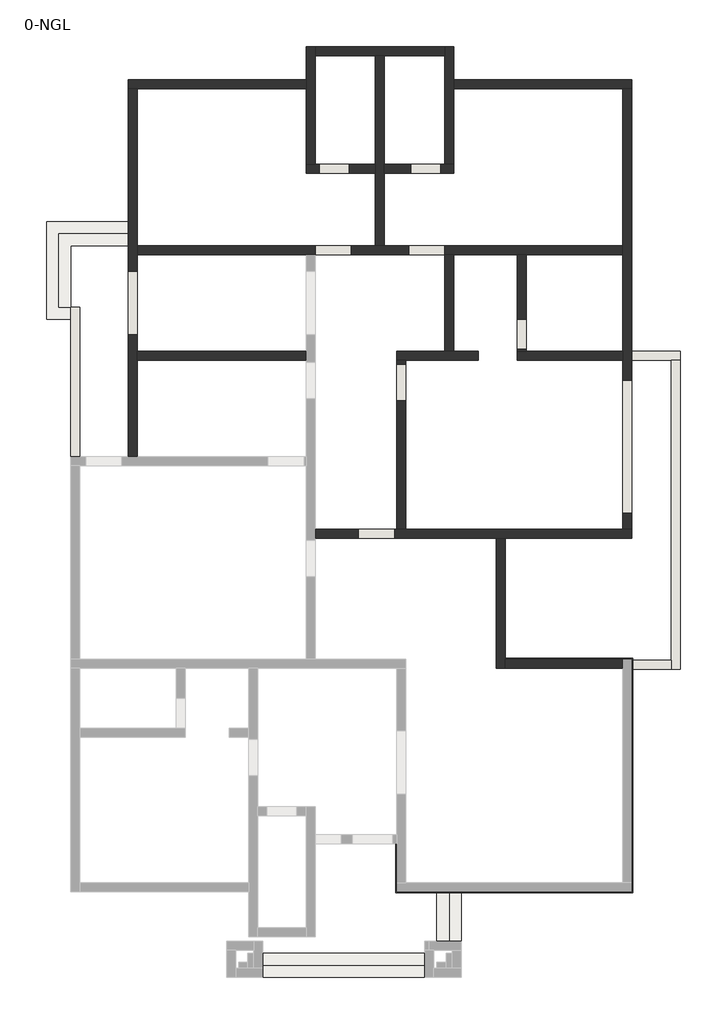
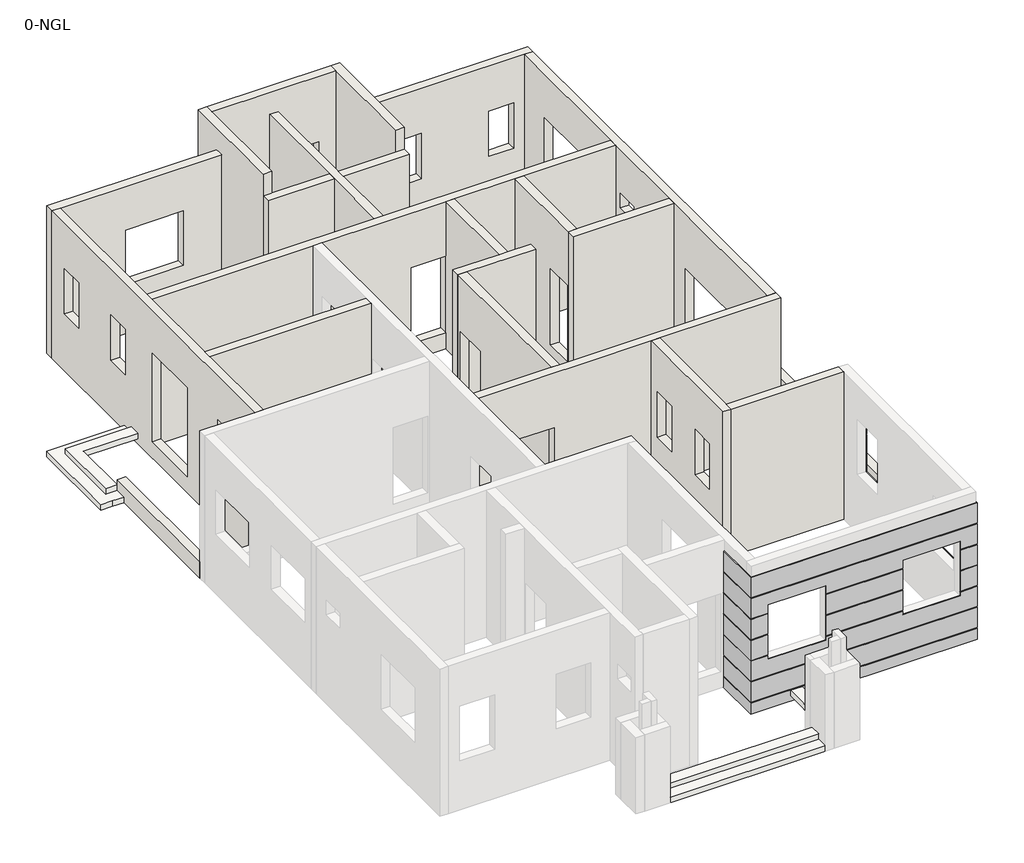
# One storey, part 2 of 2: 23 walls, 4 slabs, 1 furniture element.
"""IFC4 building model written with IfcOpenShell, lengths in millimetres."""

from ifc_helpers import new_model, si_unit, frame, origin, origin_with_axes, place, context, project, spatial, polyline, outline, extrude, faceted_brep, transform, mapped, element, save
from components import casework_8_casework_8_de918fe4

model = new_model("IFC4")

# Units and contexts
model_context = context("Model", 3, world=origin())
ifc_project = project(units=[si_unit("LENGTHUNIT", "METRE", prefix="MILLI")], contexts=[model_context])

# Site, building, storey
site = spatial("IfcSite", under=ifc_project)
building = spatial("IfcBuilding", under=site)
storey = spatial("IfcBuildingStorey", under=building, Name="0-NGL", Elevation=0.0)

# Furniture
placement = place(None, origin())
casework_8_casework_8_shape = casework_8_casework_8_de918fe4(model_context)
element("IfcFurniture", 1, ObjectType="Casework 8 : Casework 8", at=placement, inside=storey, context=model_context, shape_type="MappedRepresentation", body=[
    mapped(casework_8_casework_8_shape, transform((0.0, 0.0, 0.0), x_axis=(1.0, 0.0, 0.0), y_axis=(0.0, 1.0, 0.0), z_axis=(0.0, 0.0, 1.0))),
])

# Slabs
element("IfcSlab", 2, ObjectType="6\" floor", at=placement, inside=storey, context=model_context, shape_type="SweptSolid", body=[
    extrude(outline(polyline([(-6111.7953966, 4965.8070837), (-6111.7953966, 3440.8070837), (-6411.7953966, 3440.8070837), (-6411.7953966, 5265.8070837), (-4686.7953966, 5265.8070837), (-4686.7953966, 4965.8070837), (-6111.7953966, 4965.8070837)])), frame((0.0, 0.0, 150.0), z_axis=(0.0, 0.0, 1.0), x_axis=(1.0, 0.0, 0.0)), (0.0, 0.0, 1.0), 150.0),
])
element("IfcSlab", 3, ObjectType="6\" floor", at=placement, inside=storey, context=model_context, shape_type="SweptSolid", body=[
    extrude(outline(polyline([(-6411.7953966, 5265.8070837), (-6411.7953966, 3440.8070837), (-6111.7953966, 3440.8070837), (-6111.7953966, 3140.8070837), (-6411.7953966, 3140.8070837), (-6711.7953966, 3140.8070837), (-6711.7953966, 5565.8070837), (-4686.7953966, 5565.8070837), (-4686.7953966, 5265.8070837), (-6411.7953966, 5265.8070837)])), origin_with_axes(), (0.0, 0.0, 1.0), 150.0),
])
element("IfcSlab", 4, ObjectType="6\" floor", at=placement, inside=storey, context=model_context, shape_type="SweptSolid", body=[
    extrude(outline(polyline([(2993.2046034, -11134.1929163), (3293.2046034, -11134.1929163), (3293.2046034, -12324.1929163), (2993.2046034, -12324.1929163), (2993.2046034, -11134.1929163)])), frame((0.0, 0.0, 150.0), z_axis=(0.0, 0.0, 1.0), x_axis=(1.0, 0.0, 0.0)), (0.0, 0.0, 1.0), 150.0),
    extrude(outline(polyline([(2693.2046034, -12624.1929163), (2693.2046034, -12924.1929163), (-1336.7953966, -12924.1929163), (-1336.7953966, -12624.1929163), (2693.2046034, -12624.1929163)])), frame((0.0, 0.0, 150.0), z_axis=(0.0, 0.0, 1.0), x_axis=(1.0, 0.0, 0.0)), (0.0, 0.0, 1.0), 150.0),
])
element("IfcSlab", 5, ObjectType="6\" floor", at=placement, inside=storey, context=model_context, shape_type="SweptSolid", body=[
    extrude(outline(polyline([(3293.2046034, -11134.1929163), (3593.2046034, -11134.1929163), (3593.2046034, -12324.1929163), (3293.2046034, -12324.1929163), (3293.2046034, -11134.1929163)])), origin_with_axes(), (0.0, 0.0, 1.0), 150.0),
    extrude(outline(polyline([(2693.2046034, -12924.1929163), (2693.2046034, -13224.1929163), (-1336.7953966, -13224.1929163), (-1336.7953966, -12924.1929163), (2693.2046034, -12924.1929163)])), origin_with_axes(), (0.0, 0.0, 1.0), 150.0),
])

# Walls
element("IfcWall", 6, ObjectType="225 wall", at=placement, inside=storey, context=model_context, shape_type="Brep", body=[
    faceted_brep([(-4686.7953966, 8865.8070837, 0.0), (-4461.7953966, 8865.8070837, 0.0), (-261.7953966, 8865.8070837, 0.0), (-261.7953966, 8865.8070837, 4050.0), (-4461.7953966, 8865.8070837, 4050.0), (-4686.7953966, 8865.8070837, 4050.0), (-1261.7953966, 8865.8070837, 2850.0), (-1261.7953966, 8865.8070837, 1350.0), (-2761.7953966, 8865.8070837, 1350.0), (-2761.7953966, 8865.8070837, 2850.0), (-4686.7953966, 9090.8070837, 0.0), (-4686.7953966, 9090.8070837, 4050.0), (-261.7953966, 9090.8070837, 4050.0), (-261.7953966, 9090.8070837, 0.0), (-1261.7953966, 9090.8070837, 2850.0), (-2761.7953966, 9090.8070837, 2850.0), (-2761.7953966, 9090.8070837, 1350.0), (-1261.7953966, 9090.8070837, 1350.0)], [[[0, 1, 2, 3, 4, 5], [6, 7, 8, 9]], [[10, 11, 12, 13], [14, 15, 16, 17]], [[2, 1, 0, 10, 13]], [[5, 4, 3, 12, 11]], [[0, 5, 11, 10]], [[3, 2, 13, 12]], [[7, 6, 14, 17]], [[8, 7, 17, 16]], [[9, 8, 16, 15]], [[6, 9, 15, 14]]]),
])
element("IfcWall", 7, ObjectType="225 wall", at=placement, inside=storey, context=model_context, shape_type="Brep", body=[
    faceted_brep([(1688.2046034, 4965.8070837, 0.0), (1688.2046034, 6765.8070837, 0.0), (1688.2046034, 6990.8070837, 0.0), (1688.2046034, 9690.8070837, 0.0), (1688.2046034, 9690.8070837, 4050.0), (1688.2046034, 6990.8070837, 4050.0), (1688.2046034, 6765.8070837, 4050.0), (1688.2046034, 4965.8070837, 4050.0), (1463.2046034, 4965.8070837, 0.0), (1463.2046034, 4965.8070837, 4050.0), (1463.2046034, 6765.8070837, 4050.0), (1463.2046034, 6990.8070837, 4050.0), (1463.2046034, 9690.8070837, 4050.0), (1463.2046034, 9690.8070837, 0.0), (1463.2046034, 6990.8070837, 0.0), (1463.2046034, 6765.8070837, 0.0)], [[[0, 1, 2, 3, 4, 5, 6, 7]], [[8, 9, 10, 11, 12, 13, 14, 15]], [[3, 2, 1, 0, 8, 15, 14, 13]], [[7, 6, 5, 4, 12, 11, 10, 9]], [[4, 3, 13, 12]], [[0, 7, 9, 8]]]),
])
element("IfcWall", 8, ObjectType="225 wall", at=placement, inside=storey, context=model_context, shape_type="Brep", body=[
    faceted_brep([(-36.7953966, 9690.8070837, 0.0), (1463.2046034, 9690.8070837, 0.0), (1688.2046034, 9690.8070837, 0.0), (3188.2046034, 9690.8070837, 0.0), (3188.2046034, 9690.8070837, 4650.0), (-36.7953966, 9690.8070837, 4650.0), (2738.2046034, 9690.8070837, 2850.0), (2738.2046034, 9690.8070837, 2450.0), (2138.2046034, 9690.8070837, 2450.0), (2138.2046034, 9690.8070837, 2850.0), (1013.2046034, 9690.8070837, 2850.0), (1013.2046034, 9690.8070837, 2450.0), (413.2046034, 9690.8070837, 2450.0), (413.2046034, 9690.8070837, 2850.0), (-36.7953966, 9915.8070837, 0.0), (-36.7953966, 9915.8070837, 4650.0), (3188.2046034, 9915.8070837, 4650.0), (3188.2046034, 9915.8070837, 0.0), (2738.2046034, 9915.8070837, 2850.0), (2138.2046034, 9915.8070837, 2850.0), (2138.2046034, 9915.8070837, 2450.0), (2738.2046034, 9915.8070837, 2450.0), (1013.2046034, 9915.8070837, 2850.0), (413.2046034, 9915.8070837, 2850.0), (413.2046034, 9915.8070837, 2450.0), (1013.2046034, 9915.8070837, 2450.0)], [[[0, 1, 2, 3, 4, 5], [6, 7, 8, 9], [10, 11, 12, 13]], [[14, 15, 16, 17], [18, 19, 20, 21], [22, 23, 24, 25]], [[3, 2, 1, 0, 14, 17]], [[5, 4, 16, 15]], [[0, 5, 15, 14]], [[4, 3, 17, 16]], [[7, 6, 18, 21]], [[8, 7, 21, 20]], [[9, 8, 20, 19]], [[6, 9, 19, 18]], [[11, 10, 22, 25]], [[12, 11, 25, 24]], [[13, 12, 24, 23]], [[10, 13, 23, 22]]]),
])
element("IfcWall", 9, ObjectType="225 wall", at=placement, inside=storey, context=model_context, shape_type="Brep", body=[
    faceted_brep([(3413.2046034, 8865.8070837, 0.0), (7613.2046034, 8865.8070837, 0.0), (7838.2046034, 8865.8070837, 0.0), (7838.2046034, 8865.8070837, 4050.0), (7613.2046034, 8865.8070837, 4050.0), (3413.2046034, 8865.8070837, 4050.0), (4938.2046034, 8865.8070837, 1565.0), (4288.2046034, 8865.8070837, 1565.0), (4288.2046034, 8865.8070837, 2815.0), (4938.2046034, 8865.8070837, 2815.0), (7338.2046034, 8865.8070837, 1565.0), (6688.2046034, 8865.8070837, 1565.0), (6688.2046034, 8865.8070837, 2815.0), (7338.2046034, 8865.8070837, 2815.0), (3413.2046034, 9090.8070837, 0.0), (3413.2046034, 9090.8070837, 4050.0), (7838.2046034, 9090.8070837, 4050.0), (7838.2046034, 9090.8070837, 0.0), (4938.2046034, 9090.8070837, 1565.0), (4938.2046034, 9090.8070837, 2815.0), (4288.2046034, 9090.8070837, 2815.0), (4288.2046034, 9090.8070837, 1565.0), (7338.2046034, 9090.8070837, 1565.0), (7338.2046034, 9090.8070837, 2815.0), (6688.2046034, 9090.8070837, 2815.0), (6688.2046034, 9090.8070837, 1565.0)], [[[0, 1, 2, 3, 4, 5], [6, 7, 8, 9], [10, 11, 12, 13]], [[14, 15, 16, 17], [18, 19, 20, 21], [22, 23, 24, 25]], [[2, 1, 0, 14, 17]], [[5, 4, 3, 16, 15]], [[0, 5, 15, 14]], [[3, 2, 17, 16]], [[19, 18, 6, 9]], [[20, 19, 9, 8]], [[21, 20, 8, 7]], [[18, 21, 7, 6]], [[23, 22, 10, 13]], [[24, 23, 13, 12]], [[25, 24, 12, 11]], [[22, 25, 11, 10]]]),
])
element("IfcWall", 10, ObjectType="225 wall", at=placement, inside=storey, context=model_context, shape_type="Brep", body=[
    faceted_brep([(-261.7953966, 6765.8070837, 4050.0), (-261.7953966, 6765.8070837, 0.0), (1463.2046034, 6765.8070837, 0.0), (1463.2046034, 6765.8070837, 4050.0), (63.2046034, 6765.8070837, 450.0), (63.2046034, 6765.8070837, 2550.0), (813.2046034, 6765.8070837, 2550.0), (813.2046034, 6765.8070837, 450.0), (-261.7953966, 6990.8070837, 0.0), (-261.7953966, 6990.8070837, 4050.0), (1463.2046034, 6990.8070837, 4050.0), (1463.2046034, 6990.8070837, 0.0), (-36.7953966, 6990.8070837, 0.0), (63.2046034, 6990.8070837, 2550.0), (63.2046034, 6990.8070837, 450.0), (813.2046034, 6990.8070837, 450.0), (813.2046034, 6990.8070837, 2550.0)], [[[0, 1, 2, 3], [4, 5, 6, 7]], [[8, 9, 10, 11, 12], [13, 14, 15, 16]], [[1, 8, 12, 11, 2]], [[9, 0, 3, 10]], [[3, 2, 11, 10]], [[1, 0, 9, 8]], [[5, 4, 14, 13]], [[6, 5, 13, 16]], [[7, 6, 16, 15]], [[4, 7, 15, 14]]]),
    faceted_brep([(3413.2046034, 6765.8070837, 0.0), (3413.2046034, 6765.8070837, 4050.0), (1688.2046034, 6765.8070837, 4050.0), (1688.2046034, 6765.8070837, 0.0), (3088.2046034, 6765.8070837, 2550.0), (3088.2046034, 6765.8070837, 450.0), (2338.2046034, 6765.8070837, 450.0), (2338.2046034, 6765.8070837, 2550.0), (3413.2046034, 6990.8070837, 4050.0), (3413.2046034, 6990.8070837, 0.0), (3188.2046034, 6990.8070837, 0.0), (1688.2046034, 6990.8070837, 0.0), (1688.2046034, 6990.8070837, 4050.0), (3088.2046034, 6990.8070837, 450.0), (3088.2046034, 6990.8070837, 2550.0), (2338.2046034, 6990.8070837, 2550.0), (2338.2046034, 6990.8070837, 450.0)], [[[0, 1, 2, 3], [4, 5, 6, 7]], [[8, 9, 10, 11, 12], [13, 14, 15, 16]], [[9, 0, 3, 11, 10]], [[1, 8, 12, 2]], [[3, 2, 12, 11]], [[1, 0, 9, 8]], [[14, 13, 5, 4]], [[15, 14, 4, 7]], [[16, 15, 7, 6]], [[13, 16, 6, 5]]]),
])
element("IfcWall", 11, ObjectType="225 wall", at=placement, inside=storey, context=model_context, shape_type="Brep", body=[
    faceted_brep([(-36.7953966, 6990.8070837, 0.0), (-36.7953966, 9690.8070837, 0.0), (-36.7953966, 9915.8070837, 0.0), (-36.7953966, 9915.8070837, 4650.0), (-36.7953966, 9690.8070837, 4650.0), (-36.7953966, 6990.8070837, 4650.0), (-261.7953966, 6990.8070837, 0.0), (-261.7953966, 6990.8070837, 4050.0), (-261.7953966, 6990.8070837, 4650.0), (-261.7953966, 9915.8070837, 4650.0), (-261.7953966, 9915.8070837, 0.0), (-261.7953966, 9090.8070837, 0.0), (-261.7953966, 8865.8070837, 0.0)], [[[0, 1, 2, 3, 4, 5]], [[6, 7, 8, 9, 10, 11, 12]], [[2, 1, 0, 6, 12, 11, 10]], [[5, 4, 3, 9, 8]], [[3, 2, 10, 9]], [[0, 5, 8, 7, 6]]]),
])
element("IfcWall", 12, ObjectType="225 wall", at=placement, inside=storey, context=model_context, shape_type="Brep", body=[
    faceted_brep([(3413.2046034, 6990.8070837, 0.0), (3413.2046034, 8865.8070837, 0.0), (3413.2046034, 9090.8070837, 0.0), (3413.2046034, 9915.8070837, 0.0), (3413.2046034, 9915.8070837, 4650.0), (3413.2046034, 6990.8070837, 4650.0), (3413.2046034, 6990.8070837, 4050.0), (3188.2046034, 6990.8070837, 0.0), (3188.2046034, 6990.8070837, 4650.0), (3188.2046034, 9690.8070837, 4650.0), (3188.2046034, 9915.8070837, 4650.0), (3188.2046034, 9915.8070837, 0.0), (3188.2046034, 9690.8070837, 0.0)], [[[0, 1, 2, 3, 4, 5, 6]], [[7, 8, 9, 10, 11, 12]], [[3, 2, 1, 0, 7, 12, 11]], [[5, 4, 10, 9, 8]], [[4, 3, 11, 10]], [[0, 6, 5, 8, 7]]]),
])
element("IfcWall", 13, ObjectType="225 wall", at=placement, inside=storey, context=model_context, shape_type="SweptSolid", body=[
    extrude(outline(polyline([(-261.7953966, 2115.8070837), (-4461.7953966, 2115.8070837), (-4461.7953966, 2340.8070837), (-261.7953966, 2340.8070837), (-261.7953966, 2115.8070837)])), origin_with_axes(), (0.0, 0.0, 1.0), 4050.0),
])
element("IfcWall", 14, ObjectType="225 wall", at=placement, inside=storey, context=model_context, shape_type="Brep", body=[
    faceted_brep([(1988.2046034, 2115.8070837, 0.0), (2213.2046034, 2115.8070837, 0.0), (4013.2046034, 2115.8070837, 0.0), (4013.2046034, 2115.8070837, 4050.0), (2213.2046034, 2115.8070837, 4050.0), (1988.2046034, 2115.8070837, 4050.0), (1988.2046034, 2340.8070837, 0.0), (1988.2046034, 2340.8070837, 4050.0), (3188.2046034, 2340.8070837, 4050.0), (3413.2046034, 2340.8070837, 4050.0), (4013.2046034, 2340.8070837, 4050.0), (4013.2046034, 2340.8070837, 0.0), (3413.2046034, 2340.8070837, 0.0), (3188.2046034, 2340.8070837, 0.0)], [[[0, 1, 2, 3, 4, 5]], [[6, 7, 8, 9, 10, 11, 12, 13]], [[2, 1, 0, 6, 13, 12, 11]], [[3, 2, 11, 10]], [[5, 4, 3, 10, 9, 8, 7]], [[0, 5, 7, 6]]]),
])
element("IfcWall", 15, ObjectType="225 wall", at=placement, inside=storey, context=model_context, shape_type="Brep", body=[
    faceted_brep([(-36.7953966, -2309.1929163, 0.0), (4463.2046034, -2309.1929163, 0.0), (4688.2046034, -2309.1929163, 0.0), (7838.2046034, -2309.1929163, 0.0), (7838.2046034, -2309.1929163, 4050.0), (4688.2046034, -2309.1929163, 4050.0), (4463.2046034, -2309.1929163, 4050.0), (-36.7953966, -2309.1929163, 4050.0), (1938.2046034, -2309.1929163, 450.0), (1038.2046034, -2309.1929163, 450.0), (1038.2046034, -2309.1929163, 2550.0), (1938.2046034, -2309.1929163, 2550.0), (-36.7953966, -2084.1929163, 0.0), (-36.7953966, -2084.1929163, 4050.0), (1988.2046034, -2084.1929163, 4050.0), (2213.2046034, -2084.1929163, 4050.0), (7613.2046034, -2084.1929163, 4050.0), (7838.2046034, -2084.1929163, 4050.0), (7838.2046034, -2084.1929163, 0.0), (7613.2046034, -2084.1929163, 0.0), (2213.2046034, -2084.1929163, 0.0), (1988.2046034, -2084.1929163, 0.0), (1938.2046034, -2084.1929163, 450.0), (1938.2046034, -2084.1929163, 2550.0), (1038.2046034, -2084.1929163, 2550.0), (1038.2046034, -2084.1929163, 450.0)], [[[0, 1, 2, 3, 4, 5, 6, 7], [8, 9, 10, 11]], [[12, 13, 14, 15, 16, 17, 18, 19, 20, 21], [22, 23, 24, 25]], [[3, 2, 1, 0, 12, 21, 20, 19, 18]], [[7, 6, 5, 4, 17, 16, 15, 14, 13]], [[0, 7, 13, 12]], [[4, 3, 18, 17]], [[23, 22, 8, 11]], [[24, 23, 11, 10]], [[25, 24, 10, 9]], [[22, 25, 9, 8]]]),
])
element("IfcWall", 16, ObjectType="225 wall", at=placement, inside=storey, context=model_context, shape_type="Brep", body=[
    faceted_brep([(4688.2046034, -5534.1929163, 0.0), (4688.2046034, -5309.1929163, 0.0), (4688.2046034, -2309.1929163, 0.0), (4688.2046034, -2309.1929163, 4050.0), (4688.2046034, -5309.1929163, 4050.0), (4688.2046034, -5534.1929163, 4050.0), (4688.2046034, -2584.1929163, 1565.0), (4688.2046034, -3234.1929163, 1565.0), (4688.2046034, -3234.1929163, 2815.0), (4688.2046034, -2584.1929163, 2815.0), (4688.2046034, -4284.1929163, 1565.0), (4688.2046034, -4934.1929163, 1565.0), (4688.2046034, -4934.1929163, 2815.0), (4688.2046034, -4284.1929163, 2815.0), (4463.2046034, -5534.1929163, 0.0), (4463.2046034, -5534.1929163, 4050.0), (4463.2046034, -2309.1929163, 4050.0), (4463.2046034, -2309.1929163, 0.0), (4463.2046034, -2584.1929163, 1565.0), (4463.2046034, -2584.1929163, 2815.0), (4463.2046034, -3234.1929163, 2815.0), (4463.2046034, -3234.1929163, 1565.0), (4463.2046034, -4284.1929163, 1565.0), (4463.2046034, -4284.1929163, 2815.0), (4463.2046034, -4934.1929163, 2815.0), (4463.2046034, -4934.1929163, 1565.0)], [[[0, 1, 2, 3, 4, 5], [6, 7, 8, 9], [10, 11, 12, 13]], [[14, 15, 16, 17], [18, 19, 20, 21], [22, 23, 24, 25]], [[2, 1, 0, 14, 17]], [[5, 4, 3, 16, 15]], [[3, 2, 17, 16]], [[19, 18, 6, 9]], [[20, 19, 9, 8]], [[21, 20, 8, 7]], [[18, 21, 7, 6]], [[23, 22, 10, 13]], [[24, 23, 13, 12]], [[25, 24, 12, 11]], [[22, 25, 11, 10]], [[0, 5, 15, 14]]]),
])
element("IfcWall", 17, ObjectType="225 wall", at=placement, inside=storey, context=model_context, shape_type="SweptSolid", body=[
    extrude(outline(polyline([(-2084.1929163, 0.0), (-2084.1929163, 4050.0), (2115.8070837, 4050.0), (2115.8070837, 0.0), (-2084.1929163, 0.0)]), holes=[polyline([(2015.8070837, 450.0), (2015.8070837, 2550.0), (1115.8070837, 2550.0), (1115.8070837, 450.0), (2015.8070837, 450.0)])]), frame((1988.2046034, 0.0, 0.0), z_axis=(1.0, 0.0, 0.0), x_axis=(0.0, 1.0, 0.0)), (0.0, 0.0, 1.0), 225.0),
])
element("IfcWall", 18, ObjectType="225 wall", at=placement, inside=storey, context=model_context, shape_type="Brep", body=[
    faceted_brep([(3413.2046034, 2340.8070837, 0.0), (3413.2046034, 4740.8070837, 0.0), (3413.2046034, 4740.8070837, 4050.0), (3413.2046034, 2340.8070837, 4050.0), (3188.2046034, 2340.8070837, 0.0), (3188.2046034, 2340.8070837, 4050.0), (3188.2046034, 4740.8070837, 4050.0), (3188.2046034, 4740.8070837, 2550.0), (3188.2046034, 4740.8070837, 450.0), (3188.2046034, 4740.8070837, 0.0)], [[[0, 1, 2, 3]], [[4, 5, 6, 7, 8, 9]], [[1, 0, 4, 9]], [[3, 2, 6, 5]], [[2, 1, 9, 8, 7, 6]], [[0, 3, 5, 4]]]),
])
element("IfcWall", 19, ObjectType="225 wall", at=placement, inside=storey, context=model_context, shape_type="Brep", body=[
    faceted_brep([(-4461.7953966, -284.1929163, 0.0), (-4461.7953966, 2115.8070837, 0.0), (-4461.7953966, 2340.8070837, 0.0), (-4461.7953966, 4740.8070837, 0.0), (-4461.7953966, 4965.8070837, 0.0), (-4461.7953966, 8865.8070837, 0.0), (-4461.7953966, 8865.8070837, 4050.0), (-4461.7953966, 4965.8070837, 4050.0), (-4461.7953966, 4740.8070837, 4050.0), (-4461.7953966, 2340.8070837, 4050.0), (-4461.7953966, 2115.8070837, 4050.0), (-4461.7953966, -284.1929163, 4050.0), (-4461.7953966, 4330.8070837, 450.0), (-4461.7953966, 2750.8070837, 450.0), (-4461.7953966, 2750.8070837, 2890.0), (-4461.7953966, 4330.8070837, 2890.0), (-4461.7953966, 465.8070837, 2850.0), (-4461.7953966, 1365.8070837, 2850.0), (-4461.7953966, 1365.8070837, 1950.0), (-4461.7953966, 465.8070837, 1950.0), (-4461.7953966, 7640.8070837, 1565.0), (-4461.7953966, 7640.8070837, 2815.0), (-4461.7953966, 8290.8070837, 2815.0), (-4461.7953966, 8290.8070837, 1565.0), (-4461.7953966, 6190.8070837, 1565.0), (-4461.7953966, 5540.8070837, 1565.0), (-4461.7953966, 5540.8070837, 2815.0), (-4461.7953966, 6190.8070837, 2815.0), (-4686.7953966, -284.1929163, 0.0), (-4686.7953966, -284.1929163, 4050.0), (-4686.7953966, 8865.8070837, 4050.0), (-4686.7953966, 8865.8070837, 0.0), (-4686.7953966, 4330.8070837, 450.0), (-4686.7953966, 4330.8070837, 2890.0), (-4686.7953966, 2750.8070837, 2890.0), (-4686.7953966, 2750.8070837, 450.0), (-4686.7953966, 465.8070837, 2850.0), (-4686.7953966, 465.8070837, 1950.0), (-4686.7953966, 1365.8070837, 1950.0), (-4686.7953966, 1365.8070837, 2850.0), (-4686.7953966, 7640.8070837, 1565.0), (-4686.7953966, 8290.8070837, 1565.0), (-4686.7953966, 8290.8070837, 2815.0), (-4686.7953966, 7640.8070837, 2815.0), (-4686.7953966, 6190.8070837, 1565.0), (-4686.7953966, 6190.8070837, 2815.0), (-4686.7953966, 5540.8070837, 2815.0), (-4686.7953966, 5540.8070837, 1565.0)], [[[0, 1, 2, 3, 4, 5, 6, 7, 8, 9, 10, 11], [12, 13, 14, 15], [16, 17, 18, 19], [20, 21, 22, 23], [24, 25, 26, 27]], [[28, 29, 30, 31], [32, 33, 34, 35], [36, 37, 38, 39], [40, 41, 42, 43], [44, 45, 46, 47]], [[5, 4, 3, 2, 1, 0, 28, 31]], [[11, 10, 9, 8, 7, 6, 30, 29]], [[6, 5, 31, 30]], [[0, 11, 29, 28]], [[33, 32, 12, 15]], [[34, 33, 15, 14]], [[35, 34, 14, 13]], [[32, 35, 13, 12]], [[37, 36, 16, 19]], [[38, 37, 19, 18]], [[39, 38, 18, 17]], [[36, 39, 17, 16]], [[21, 20, 40, 43]], [[22, 21, 43, 42]], [[23, 22, 42, 41]], [[20, 23, 41, 40]], [[45, 44, 24, 27]], [[46, 45, 27, 26]], [[47, 46, 26, 25]], [[44, 47, 25, 24]]]),
])
element("IfcWall", 20, ObjectType="225 wall", at=placement, inside=storey, context=model_context, shape_type="Brep", body=[
    faceted_brep([(8813.2046034, 2115.8070837, 0.0), (8813.2046034, -5334.1929163, 0.0), (8813.2046034, -5559.1929163, 0.0), (8813.2046034, -5559.1929163, 450.0), (8813.2046034, -5334.1929163, 450.0), (8813.2046034, 2115.8070837, 450.0), (9038.2046034, 2115.8070837, 0.0), (9038.2046034, 2115.8070837, 450.0), (9038.2046034, -5559.1929163, 450.0), (9038.2046034, -5559.1929163, 0.0)], [[[0, 1, 2, 3, 4, 5]], [[6, 7, 8, 9]], [[2, 1, 0, 6, 9]], [[5, 4, 3, 8, 7]], [[0, 5, 7, 6]], [[3, 2, 9, 8]]]),
])
element("IfcWall", 21, ObjectType="225 wall", at=placement, inside=storey, context=model_context, shape_type="Brep", body=[
    faceted_brep([(7838.2046034, -2084.1929163, 0.0), (7838.2046034, 2115.8070837, 0.0), (7838.2046034, 2340.8070837, 0.0), (7838.2046034, 8865.8070837, 0.0), (7838.2046034, 8865.8070837, 4050.0), (7838.2046034, -2084.1929163, 4050.0), (7838.2046034, 3940.8070837, 2850.0), (7838.2046034, 4540.8070837, 2850.0), (7838.2046034, 4540.8070837, 2450.0), (7838.2046034, 3940.8070837, 2450.0), (7838.2046034, 7965.8070837, 2850.0), (7838.2046034, 7965.8070837, 1350.0), (7838.2046034, 6465.8070837, 1350.0), (7838.2046034, 6465.8070837, 2850.0), (7838.2046034, 1615.8070837, 2550.0), (7838.2046034, 1615.8070837, 450.0), (7838.2046034, -1684.1929163, 450.0), (7838.2046034, -1684.1929163, 2550.0), (7613.2046034, 8865.8070837, 0.0), (7613.2046034, 4965.8070837, 0.0), (7613.2046034, 4740.8070837, 0.0), (7613.2046034, 2340.8070837, 0.0), (7613.2046034, 2115.8070837, 0.0), (7613.2046034, -2084.1929163, 0.0), (7613.2046034, -2084.1929163, 4050.0), (7613.2046034, 2115.8070837, 4050.0), (7613.2046034, 2340.8070837, 4050.0), (7613.2046034, 4740.8070837, 4050.0), (7613.2046034, 4965.8070837, 4050.0), (7613.2046034, 8865.8070837, 4050.0), (7613.2046034, 3940.8070837, 2850.0), (7613.2046034, 3940.8070837, 2450.0), (7613.2046034, 4540.8070837, 2450.0), (7613.2046034, 4540.8070837, 2850.0), (7613.2046034, 7965.8070837, 2850.0), (7613.2046034, 6465.8070837, 2850.0), (7613.2046034, 6465.8070837, 1350.0), (7613.2046034, 7965.8070837, 1350.0), (7613.2046034, 1615.8070837, 450.0), (7613.2046034, 1615.8070837, 2550.0), (7613.2046034, -1684.1929163, 2550.0), (7613.2046034, -1684.1929163, 450.0)], [[[0, 1, 2, 3, 4, 5], [6, 7, 8, 9], [10, 11, 12, 13], [14, 15, 16, 17]], [[18, 19, 20, 21, 22, 23, 24, 25, 26, 27, 28, 29], [30, 31, 32, 33], [34, 35, 36, 37], [38, 39, 40, 41]], [[3, 2, 1, 0, 23, 22, 21, 20, 19, 18]], [[5, 4, 29, 28, 27, 26, 25, 24]], [[4, 3, 18, 29]], [[0, 5, 24, 23]], [[31, 30, 6, 9]], [[32, 31, 9, 8]], [[33, 32, 8, 7]], [[30, 33, 7, 6]], [[11, 10, 34, 37]], [[12, 11, 37, 36]], [[13, 12, 36, 35]], [[10, 13, 35, 34]], [[38, 15, 14, 39]], [[39, 14, 17, 40]], [[40, 17, 16, 41]], [[15, 38, 41, 16]]]),
])
element("IfcWall", 22, ObjectType="225 wall", at=placement, inside=storey, context=model_context, shape_type="Brep", body=[
    faceted_brep([(7838.2046034, 2115.8070837, 0.0), (8813.2046034, 2115.8070837, 0.0), (9038.2046034, 2115.8070837, 0.0), (9038.2046034, 2115.8070837, 450.0), (8813.2046034, 2115.8070837, 450.0), (7838.2046034, 2115.8070837, 450.0), (7838.2046034, 2340.8070837, 0.0), (7838.2046034, 2340.8070837, 450.0), (9038.2046034, 2340.8070837, 450.0), (9038.2046034, 2340.8070837, 0.0)], [[[0, 1, 2, 3, 4, 5]], [[6, 7, 8, 9]], [[2, 1, 0, 6, 9]], [[5, 4, 3, 8, 7]], [[3, 2, 9, 8]], [[0, 5, 7, 6]]]),
])
element("IfcWall", 23, ObjectType="225 wall", at=placement, inside=storey, context=model_context, shape_type="SweptSolid", body=[
    extrude(outline(polyline([(7838.2046034, -5334.1929163), (8813.2046034, -5334.1929163), (8813.2046034, -5559.1929163), (7838.2046034, -5559.1929163), (7838.2046034, -5334.1929163)])), origin_with_axes(), (0.0, 0.0, 1.0), 450.0),
])
element("IfcWall", 24, ObjectType="225 wall", at=placement, inside=storey, context=model_context, shape_type="Brep", body=[
    faceted_brep([(-4461.7953966, 4740.8070837, 0.0), (-261.7953966, 4740.8070837, 0.0), (-36.7953966, 4740.8070837, 0.0), (3188.2046034, 4740.8070837, 0.0), (3413.2046034, 4740.8070837, 0.0), (4988.2046034, 4740.8070837, 0.0), (5213.2046034, 4740.8070837, 0.0), (7613.2046034, 4740.8070837, 0.0), (7613.2046034, 4740.8070837, 4050.0), (5213.2046034, 4740.8070837, 4050.0), (4988.2046034, 4740.8070837, 4050.0), (3413.2046034, 4740.8070837, 4050.0), (3188.2046034, 4740.8070837, 4050.0), (-36.7953966, 4740.8070837, 4050.0), (-261.7953966, 4740.8070837, 4050.0), (-4461.7953966, 4740.8070837, 4050.0), (863.2046034, 4740.8070837, 450.0), (-36.7953966, 4740.8070837, 450.0), (-36.7953966, 4740.8070837, 2550.0), (863.2046034, 4740.8070837, 2550.0), (2288.2046034, 4740.8070837, 450.0), (2288.2046034, 4740.8070837, 2550.0), (3188.2046034, 4740.8070837, 2550.0), (3188.2046034, 4740.8070837, 450.0), (-4461.7953966, 4965.8070837, 0.0), (-4461.7953966, 4965.8070837, 4050.0), (1463.2046034, 4965.8070837, 4050.0), (1688.2046034, 4965.8070837, 4050.0), (7613.2046034, 4965.8070837, 4050.0), (7613.2046034, 4965.8070837, 0.0), (1688.2046034, 4965.8070837, 0.0), (1463.2046034, 4965.8070837, 0.0), (863.2046034, 4965.8070837, 450.0), (863.2046034, 4965.8070837, 2550.0), (-36.7953966, 4965.8070837, 2550.0), (-36.7953966, 4965.8070837, 450.0), (2288.2046034, 4965.8070837, 450.0), (3188.2046034, 4965.8070837, 450.0), (3188.2046034, 4965.8070837, 2550.0), (2288.2046034, 4965.8070837, 2550.0)], [[[0, 1, 2, 3, 4, 5, 6, 7, 8, 9, 10, 11, 12, 13, 14, 15], [16, 17, 18, 19], [20, 21, 22, 23]], [[24, 25, 26, 27, 28, 29, 30, 31], [32, 33, 34, 35], [36, 37, 38, 39]], [[7, 6, 5, 4, 3, 2, 1, 0, 24, 31, 30, 29]], [[15, 14, 13, 12, 11, 10, 9, 8, 28, 27, 26, 25]], [[8, 7, 29, 28]], [[33, 32, 16, 19]], [[34, 33, 19, 18]], [[35, 34, 18, 17]], [[32, 35, 17, 16]], [[21, 20, 36, 39]], [[22, 21, 39, 38]], [[23, 22, 38, 37]], [[20, 23, 37, 36]], [[0, 15, 25, 24]]]),
])
element("IfcWall", 25, ObjectType="225 wall", at=placement, inside=storey, context=model_context, shape_type="SweptSolid", body=[
    extrude(outline(polyline([(-5886.7953966, 3440.8070837), (-5886.7953966, -284.1929163), (-6111.7953966, -284.1929163), (-6111.7953966, 3440.8070837), (-5886.7953966, 3440.8070837)])), origin_with_axes(), (0.0, 0.0, 1.0), 450.0),
])
element("IfcWall", 26, ObjectType="225 wall", at=placement, inside=storey, context=model_context, shape_type="SweptSolid", body=[
    extrude(outline(polyline([(2340.8070837, 0.0), (2340.8070837, 4050.0), (4740.8070837, 4050.0), (4740.8070837, 0.0), (2340.8070837, 0.0)]), holes=[polyline([(2390.8070837, 450.0), (3140.8070837, 450.0), (3140.8070837, 2550.0), (2390.8070837, 2550.0), (2390.8070837, 450.0)])]), frame((4988.2046034, 0.0, 0.0), z_axis=(1.0, 0.0, 0.0), x_axis=(0.0, 1.0, 0.0)), (0.0, 0.0, 1.0), 225.0),
])
element("IfcWall", 27, ObjectType="225 wall", at=placement, inside=storey, context=model_context, shape_type="Brep", body=[
    faceted_brep([(4988.2046034, 2115.8070837, 0.0), (7613.2046034, 2115.8070837, 0.0), (7613.2046034, 2115.8070837, 4050.0), (4988.2046034, 2115.8070837, 4050.0), (4988.2046034, 2340.8070837, 0.0), (4988.2046034, 2340.8070837, 4050.0), (5213.2046034, 2340.8070837, 4050.0), (7613.2046034, 2340.8070837, 4050.0), (7613.2046034, 2340.8070837, 0.0), (5213.2046034, 2340.8070837, 0.0)], [[[0, 1, 2, 3]], [[4, 5, 6, 7, 8, 9]], [[1, 0, 4, 9, 8]], [[3, 2, 7, 6, 5]], [[0, 3, 5, 4]], [[2, 1, 8, 7]]]),
])
element("IfcWall", 28, ObjectType="225 wall", at=placement, inside=storey, context=model_context, shape_type="SweptSolid", body=[
    extrude(outline(polyline([(7613.2046034, -5534.1929163), (4688.2046034, -5534.1929163), (4688.2046034, -5309.1929163), (7613.2046034, -5309.1929163), (7613.2046034, -5534.1929163)])), origin_with_axes(), (0.0, 0.0, 1.0), 4050.0),
])

save(model, "model.ifc")

# Revit data of these elements
# Type "6\" floor"
#   Function = 0
#   Layers, outside or top first: 150 mm no material (function 1)
# Type "225 wall"
#   Layers, outside or top first: 225 mm "Concrete, Cast In Situ" (function 1)
# Element 1 (IfcFurniture, "Casework 8 : Casework 8")
#   Phase Created = New Construction
# Element 2 (IfcSlab, "6\" floor")
#   built-in parameter 1001955 = 3.14159 (stored number, unit not read)
#   Height Offset From Level = 300 mm
#   Phase Created = New Construction
#   Materials on its faces: "Default Floor"
# Element 3 (IfcSlab, "6\" floor")
#   built-in parameter 1001955 = 3.14159 (stored number, unit not read)
#   Height Offset From Level = 150 mm
#   Phase Created = New Construction
#   Materials on its faces: "Default Floor"
# Element 4 (IfcSlab, "6\" floor")
#   built-in parameter 1001955 = -1.5708 (stored number, unit not read)
#   Height Offset From Level = 300 mm
#   Phase Created = New Construction
#   Materials on its faces: "Default Floor"
# Element 5 (IfcSlab, "6\" floor")
#   Height Offset From Level = 150 mm
#   Phase Created = New Construction
#   Materials on its faces: "Default Floor"
# Elements 6, 7, 9, 10, 13, 14, 15, 16, 17, 18, 19, 21, 24, 26, 27, 28 (IfcWall, "225 wall")
#   Top Offset = 0 mm
#   Base Offset = 0 mm
#   wall height = 4050 mm
#   Phase Created = New Construction
#   Base Constraint = 0-NGL
#   Top Constraint = 3-ROOF
#   Materials on its faces: "Concrete, Cast In Situ"
# Elements 8, 11, 12 (IfcWall, "225 wall")
#   Top Offset = 600 mm
#   Base Offset = 0 mm
#   wall height = 4650 mm
#   Phase Created = New Construction
#   Base Constraint = 0-NGL
#   Top Constraint = 3-ROOF
#   Materials on its faces: "Concrete, Cast In Situ"
# Elements 20, 22, 23, 25 (IfcWall, "225 wall")
#   Top Offset = 0 mm
#   Base Offset = 0 mm
#   wall height = 450 mm
#   Phase Created = New Construction
#   Base Constraint = 0-NGL
#   Top Constraint = 01-DPC
#   Materials on its faces: "Concrete, Cast In Situ"
# Materials
#   "Concrete, Cast In Situ": class "Concrete", colour RGB 191 178 173, transparency 0, Description = "physical material", Cost = 0
#   "Default Floor": colour RGB 127 127 127, transparency 0, Cost = 0
